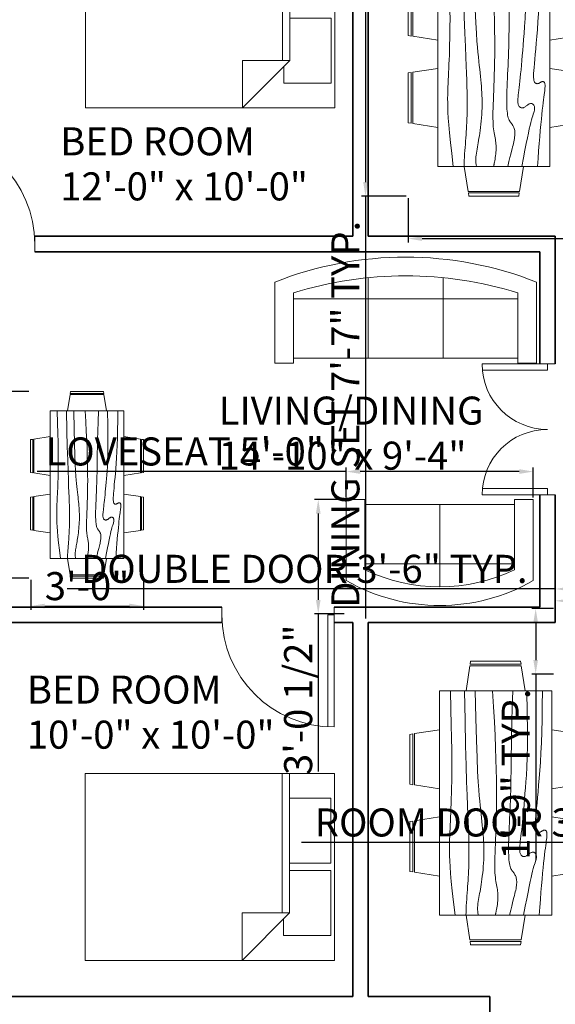
# Model space of a CAD drawing. Units: inches. Extents: x 3087 to 8148, y 1377 to 3709.
# Tile 3 of 6: x 3271 to 3443, y 1561 to 1877. Entities that reach past the tile are written whole.
import ezdxf

# ---------------------------------------------------------------- set-up
doc = ezdxf.new("R2010")
doc.units = ezdxf.units.IN
for name, color, linetype, lineweight, true_color in [('A-ANNO-DIMS', 244, 'Continuous', 18, 0x991b1e), ('A-AREA-IDEN', 244, 'Continuous', 18, 0x991b1e), ('A-DOOR', 146, 'Continuous', 18, 0x105689), ('A-WALL', 241, 'Continuous', 35, 0xf7abae)]:
    doc.layers.add(name, color=color, linetype=linetype, lineweight=lineweight, true_color=true_color)
doc.layers.add('A-FURN', color=8, linetype='Continuous', lineweight=18)
doc.styles.get("Standard").update_dxf_attribs({"font": 'arial.ttf'})
doc.dimstyles.new('ISO-25', dxfattribs={"dimtxt": 9, "dimasz": 4.5, "dimexe": 1.25, "dimexo": 0.625, "dimtad": 1, "dimdec": 0, "dimlunit": 3, "dimtxsty": 'Standard', "dimcen": 2.5, "dimadec": 0, "dimazin": 0, "dimtfac": 1, "dimtdec": 0, "dimtmove": 0, "dimatfit": 3, "dimfxl": 1, "dimarcsym": 0})

# ---------------------------------------------------------------- blocks, each defined once
blk = doc.blocks.new('Bed - Queen')
for p, q in [((0, -80.00003), (0, 0)), ((0, 0), (59.99999, 0)), ((59.99999, 0), (59.99999, -80.00003)), ((7.99999, -1.2), (28.79998, -1.2)), ((7.99999, -14.4), (7.99999, -1.2)), ((28.79998, -1.2), (28.79998, -14.4)), ((31.19999, -1.2), (51.99999, -1.2)), ((31.19999, -14.4), (31.19999, -1.2)), ((51.99999, -1.2), (51.99999, -16.4)), ((0, -14.4), (44.8, -14.4)), ((59.99999, -29.6), (44.8, -14.4)), ((44.8, -14.4), (44.8, -29.6)), ((44.8, -16.8), (0, -16.8)), ((51.99999, -16.4), (46.79936, -16.4)), ((44.8, -29.6), (59.99999, -29.6)), ((59.99999, -80.00003), (0, -80.00003))]:
    blk.add_line(p, q)
blk = doc.blocks.new('Dining Set - 36 x 72 in.')
for p, q in [((-22.2343, 26.00059), (-23.4847, 17.99762)), ((-22.2304, 26), (-5.7608, 26)), ((-22, 27.5), (-22.1562, 26.50042)), ((-5.8416, 26.5), (-22.1534, 26.5)), ((-22, 27.5), (-6, 27.5)), ((-5.8437, 26.49966), (-6, 27.5)), ((-4.5152, 17.99762), (-5.7655, 25.99926)), ((5.7657, 26.00059), (4.5153, 17.99762)), ((5.7696, 26), (22.2392, 26)), ((6, 27.5), (5.8438, 26.50042)), ((22.1584, 26.5), (5.8466, 26.5)), ((6, 27.5), (22, 27.5)), ((22.1563, 26.49966), (22, 27.5)), ((23.4848, 17.99762), (22.2345, 25.99926)), ((36, 18), (-36, 18)), ((-36, 18), (-36, -18)), ((36, -18), (36, 18)), ((-44.0006, 8.23428), (-35.9976, 9.48474)), ((44.0006, 8.23428), (35.9976, 9.48474)), ((-45.5, 8), (-44.5004, 8.15617)), ((-45.5, 8), (-45.5, -8)), ((-44.5, -8.15843), (-44.5, 8.15338)), ((-44, 8.23041), (-44, -8.23915)), ((44, 8.23041), (44, -8.23915)), ((44.5, -8.15843), (44.5, 8.15338)), ((45.5, 8), (44.5005, 8.15617)), ((45.5, 8), (45.5, -8)), ((-44.4997, -8.15631), (-45.5, -8)), ((-35.9976, -9.48476), (-43.9993, -8.2345)), ((35.9976, -9.48476), (43.9993, -8.2345)), ((44.4997, -8.15631), (45.5, -8)), ((-36, -18), (36, -18)), ((-22.2343, -26.0006), (-23.4847, -17.99762)), ((-4.5152, -17.99762), (-5.7655, -25.99928)), ((5.7657, -26.0006), (4.5153, -17.99762)), ((23.4848, -17.99762), (22.2345, -25.99928)), ((-22.2304, -26), (-5.7608, -26)), ((-22, -27.5), (-22.1562, -26.50044)), ((-5.8416, -26.5), (-22.1534, -26.5)), ((-22, -27.5), (-6, -27.5)), ((-5.8437, -26.49967), (-6, -27.5)), ((5.7696, -26), (22.2392, -26)), ((6, -27.5), (5.8438, -26.50044)), ((22.1584, -26.5), (5.8466, -26.5)), ((6, -27.5), (22, -27.5)), ((22.1563, -26.49967), (22, -27.5))]:
    blk.add_line(p, q)
for points in [[(-36, 15), (-31.1772, 14.97754), (-26.8079, 14.91406), (-22.8538, 14.81543), (-19.276, 14.6875), (-16.0362, 14.53613), (-13.0957, 14.36718), (-10.4159, 14.18652), (-7.9583, 14), (-5.6904, 13.81315), (-3.6035, 13.63021), (-1.6954, 13.45508), (0.0365, 13.29166), (1.5945, 13.14388), (2.9811, 13.01562), (4.1988, 12.9108), (5.25, 12.83333), (6.1393, 12.78613), (6.8802, 12.76823), (7.4883, 12.77767), (7.9792, 12.8125), (8.3685, 12.87077), (8.6719, 12.95052), (8.9049, 13.0498), (9.0833, 13.16666), (9.2205, 13.29899), (9.3216, 13.44401), (9.3895, 13.59879), (9.4271, 13.76041), (9.4373, 13.92594), (9.4232, 14.09245), (9.3875, 14.257), (9.3333, 14.41666), (9.2638, 14.56917), (9.1836, 14.71484), (9.0975, 14.85465), (9.0104, 14.98958), (8.9272, 15.1206), (8.8529, 15.2487), (8.7922, 15.37483), (8.75, 15.5), (8.7305, 15.62467), (8.7344, 15.74739), (8.7617, 15.86621), (8.8125, 15.97916), (8.8867, 16.08431), (8.9844, 16.17968), (9.1055, 16.26334), (9.25, 16.33333), (9.4189, 16.38802), (9.6172, 16.42708), (9.8506, 16.45052), (10.125, 16.45833), (10.4463, 16.45052), (10.8203, 16.42708), (11.2529, 16.38802), (11.75, 16.33333), (12.3184, 16.26318), (12.9694, 16.17838), (13.7151, 16.07991), (14.5677, 15.96875), (15.5395, 15.84586), (16.6426, 15.71224), (17.8893, 15.56884), (19.2917, 15.41666), (20.859, 15.25667), (22.5879, 15.08984), (24.4721, 14.91715), (26.5052, 14.73958), (28.6809, 14.5581), (30.9929, 14.3737), (33.4347, 14.18733), (36, 14)], [(-36, 10), (-28.9766, 10.14274), (-23.1725, 10.20442), (-18.4241, 10.19775), (-14.5677, 10.13541), (-11.4399, 10.03011), (-8.877, 9.89453), (-6.7154, 9.74137), (-4.7917, 9.58333), (-2.9698, 9.43082), (-1.2246, 9.28515), (0.4415, 9.14534), (2.026, 9.01041), (3.5266, 8.87939), (4.9408, 8.7513), (6.266, 8.62516), (7.5, 8.5), (8.6411, 8.37549), (9.6914, 8.2539), (10.6538, 8.13818), (11.5312, 8.03125), (12.3267, 7.93603), (13.043, 7.85547), (13.6831, 7.79248), (14.25, 7.75), (14.7471, 7.7303), (15.1797, 7.73307), (15.5537, 7.75732), (15.875, 7.80208), (16.1494, 7.86637), (16.3828, 7.94922), (16.5811, 8.04964), (16.75, 8.16666), (16.8944, 8.29915), (17.0143, 8.44531), (17.1089, 8.60319), (17.1771, 8.77083), (17.218, 8.94629), (17.2305, 9.1276), (17.2137, 9.31282), (17.1667, 9.5), (17.0895, 9.6875), (16.987, 9.875), (16.8649, 10.0625), (16.7292, 10.25), (16.5856, 10.4375), (16.4401, 10.625), (16.2985, 10.8125), (16.1667, 11), (16.05, 11.18733), (15.9518, 11.3737), (15.8752, 11.5581), (15.8229, 11.73958), (15.798, 11.91715), (15.8034, 12.08984), (15.842, 12.25667), (15.9167, 12.41666), (16.0295, 12.56836), (16.1784, 12.70833), (16.3605, 12.83268), (16.5729, 12.9375), (16.8127, 13.01888), (17.0768, 13.07291), (17.3625, 13.0957), (17.6667, 13.08333), (17.9894, 13.03312), (18.3418, 12.94726), (18.7382, 12.82918), (19.1927, 12.68229), (19.7195, 12.51001), (20.3327, 12.31575), (21.0465, 12.10294), (21.875, 11.875), (22.8357, 11.63354), (23.959, 11.37304), (25.2786, 11.08618), (26.8282, 10.76562), (28.6414, 10.40405), (30.752, 9.99414), (33.1936, 9.52856), (36, 9)], [(-36, 5.5), (-30.7157, 5.3348), (-26.069, 5.20963), (-21.9946, 5.11767), (-18.4271, 5.05208), (-15.3009, 5.00602), (-12.5508, 4.97265), (-10.1112, 4.94515), (-7.9167, 4.91666), (-5.909, 4.88167), (-4.0586, 4.83984), (-2.3429, 4.79215), (-0.7396, 4.73958), (0.7739, 4.6831), (2.22, 4.6237), (3.6213, 4.56233), (5, 4.5), (6.373, 4.43782), (7.7344, 4.3776), (9.0723, 4.32129), (10.375, 4.27083), (11.6309, 4.22819), (12.8281, 4.19531), (13.9551, 4.17415), (15, 4.16666), (15.954, 4.17448), (16.819, 4.19791), (17.6001, 4.23698), (18.3021, 4.29166), (18.9299, 4.36198), (19.4883, 4.44791), (19.9823, 4.54948), (20.4167, 4.66666), (20.7969, 4.79899), (21.1302, 4.94401), (21.4245, 5.09879), (21.6875, 5.26041), (21.9271, 5.42594), (22.1511, 5.59245), (22.3672, 5.757), (22.5834, 5.91666), (22.8065, 6.06868), (23.0404, 6.21093), (23.2879, 6.34147), (23.5521, 6.45833), (23.8358, 6.55957), (24.142, 6.64323), (24.4735, 6.70735), (24.8334, 6.75), (25.2235, 6.76969), (25.642, 6.76692), (26.0858, 6.74267), (26.5521, 6.69791), (27.0379, 6.63362), (27.5404, 6.55078), (28.0565, 6.45036), (28.5834, 6.33333), (29.1242, 6.19987), (29.7071, 6.04687), (30.3661, 5.87044), (31.1354, 5.66666), (32.0493, 5.43164), (33.142, 5.16146), (34.4475, 4.85221), (36, 4.5)], [(-36, -1), (-30.7915, -0.6591), (-26.0195, -0.38216), (-21.6519, -0.16284), (-17.6563, 0.00521), (-14.0005, 0.12833), (-10.6523, 0.21289), (-7.5796, 0.26522), (-4.75, 0.29166), (-2.134, 0.29793), (0.2878, 0.28711), (2.5317, 0.26163), (4.6146, 0.22396), (6.5529, 0.17651), (8.3633, 0.12174), (10.0623, 0.06209), (11.6667, 0), (13.1899, -0.06201), (14.6341, -0.1211), (15.9982, -0.17432), (17.2813, -0.21875), (18.4823, -0.25147), (19.6003, -0.26953), (20.6343, -0.27002), (21.5834, -0.25), (22.4481, -0.20768), (23.2357, -0.14584), (23.9549, -0.06836), (24.6146, 0.02083), (25.2235, 0.11784), (25.7904, 0.21875), (26.3241, 0.31966), (26.8334, 0.41666), (27.3265, 0.50618), (27.8099, 0.58593), (28.2894, 0.65397), (28.7709, 0.70833), (29.2601, 0.74707), (29.763, 0.76823), (30.2855, 0.76985), (30.8334, 0.75), (31.4088, 0.70784), (31.9994, 0.64713), (32.589, 0.57275), (33.1615, 0.48958), (33.7008, 0.4025), (34.1908, 0.3164), (34.6153, 0.23616), (34.9584, 0.16666), (35.2099, 0.11165), (35.3848, 0.07031), (35.504, 0.04069), (35.5886, 0.02083), (35.6594, 0.00879), (35.7377, 0.0026), (35.8442, 0.00032), (36, 0)], [(-36, -6.5), (-27.1843, -6.31267), (-20.084, -6.1263), (-14.469, -5.9419), (-10.1094, -5.76042), (-6.7752, -5.58285), (-4.2363, -5.41016), (-2.2629, -5.24333), (-0.625, -5.08334), (0.8708, -4.93099), (2.2715, -4.78646), (3.5872, -4.64974), (4.8281, -4.52084), (6.0046, -4.39974), (7.127, -4.28646), (8.2053, -4.18099), (9.25, -4.08334), (10.2705, -3.99382), (11.2734, -3.91407), (12.2647, -3.84603), (13.25, -3.79167), (14.2354, -3.75293), (15.2266, -3.73177), (16.2295, -3.73015), (17.25, -3.75), (18.2912, -3.79248), (19.3451, -3.85547), (20.4009, -3.93604), (21.4479, -4.03125), (22.4754, -4.13819), (23.4727, -4.25391), (24.4289, -4.37549), (25.3334, -4.5), (26.1785, -4.62492), (26.9694, -4.74935), (27.7145, -4.87281), (28.4219, -4.99479), (29.1, -5.11483), (29.7572, -5.23242), (30.4016, -5.34709), (31.0417, -5.45834), (31.6837, -5.56437), (32.3262, -5.65821), (32.9658, -5.73153), (33.599, -5.77604), (34.2224, -5.78345), (34.8327, -5.74545), (35.4264, -5.65373), (36, -5.5)], [(-36, -10), (-26.4022, -9.81299), (-18.4675, -9.62891), (-11.9839, -9.45069), (-6.7396, -9.28125), (-2.5226, -9.12354), (0.8789, -8.98047), (3.6769, -8.85498), (6.0833, -8.75), (8.2767, -8.66765), (10.3021, -8.60677), (12.1712, -8.56543), (13.8958, -8.54167), (15.4876, -8.53353), (16.9583, -8.53907), (18.3197, -8.55632), (19.5834, -8.58334), (20.7616, -8.61841), (21.8685, -8.66081), (22.9188, -8.71004), (23.9271, -8.76563), (24.9081, -8.82707), (25.8763, -8.89388), (26.8465, -8.96558), (27.8334, -9.04167), (28.8474, -9.12118), (29.8828, -9.20117), (30.93, -9.27824), (31.9792, -9.34896), (33.0205, -9.40991), (34.0443, -9.45768), (35.0407, -9.48885), (36, -9.5)], [(-36, -14.5), (-30.0881, -14.33513), (-25.0332, -14.21224), (-20.7312, -14.12647), (-17.0781, -14.07292), (-13.97, -14.04671), (-11.3027, -14.04297), (-8.9724, -14.05681), (-6.875, -14.08334), (-4.9224, -14.11833), (-3.0905, -14.16016), (-1.3709, -14.20785), (0.2448, -14.26042), (1.7647, -14.3169), (3.1973, -14.3763), (4.5507, -14.43767), (5.8333, -14.5), (7.0554, -14.5621), (8.235, -14.62175), (9.3922, -14.67652), (10.5469, -14.72396), (11.7192, -14.76164), (12.929, -14.78711), (14.1965, -14.79794), (15.5417, -14.79167), (16.9933, -14.76424), (18.6152, -14.70508), (20.4804, -14.60197), (22.6615, -14.44271), (25.2312, -14.21509), (28.2624, -13.9069), (31.8277, -13.50594), (36, -13)]]:
    blk.add_lwpolyline(points)
blk = doc.blocks.new('Sofa - Roundback 7 ft.')
for p, q in [((-12.00002, -32.4421), (-12.00003, -6.5971)), ((11.99997, -32.4421), (11.99998, -6.5971)), ((-36.000027, -34), (-36.000027, -11.4696)), ((35.99998, -34), (35.99998, -11.4696)), ((-35.999844, -13.3819), (35.9998, -13.3819)), ((-36.000027, -32.4421), (35.99998, -32.4421))]:
    blk.add_line(p, q)
for points in [[(-36.000027, -34), (-42.000027, -34), (-42.000027, -8)], [(41.99998, -8), (41.99998, -34), (35.99998, -34)]]:
    blk.add_lwpolyline(points)
for centre, radius, start, end in [((0, -114.25), 114.25, 68.43141, 111.5686), ((-0.00001, -127.1968), 121.1968, 72.72033, 107.2797)]:
    blk.add_arc(centre, radius, start, end)
blk = doc.blocks.new('Sofa - Roundback Loveseat 5 ft.')
for p, q in [((0, -32.44198), (0, -5.99998)), ((-24, -33.99998), (-24, -11.46958)), ((24.00004, -33.99998), (24.00004, -11.46958)), ((-23.9998, -13.38178), (23.99986, -13.38178)), ((-24, -32.44198), (24.00004, -32.44198))]:
    blk.add_line(p, q)
for points in [[(-24, -33.99998), (-30, -33.99998), (-30, -7.99998)], [(30.00004, -7.99998), (30.00004, -33.99998), (24.00004, -33.99998)]]:
    blk.add_lwpolyline(points)
for centre, radius, start, end in [((0, -60.24998), 60.24998, 60.13715, 119.8628), ((0, -61.38438), 55.38444, 64.32083, 115.6792)]:
    blk.add_arc(centre, radius, start, end)
blk = doc.blocks.new('*D19')
at = {"layer": 'A-ANNO-DIMS', "color": 0, "lineweight": -2, "transparency": 16777216}
for p, q in [((3442.82, 1703.84), (3442.82, 1689.71)), ((3630.82, 1703.84), (3630.82, 1689.71)), ((3447.32, 1690.96), (3626.32, 1690.96))]:
    blk.add_line(p, q, dxfattribs=at)
at = {"layer": 'A-ANNO-DIMS', "color": 0, "transparency": 16777216}
for points in [[(3447.32, 1691.71), (3447.32, 1690.21), (3442.82, 1690.96)], [(3626.32, 1691.71), (3626.32, 1690.21), (3630.82, 1690.96)]]:
    blk.add_solid(points, dxfattribs=at)
at = {"layer": 'Defpoints', "color": 0, "transparency": 16777216}
for p in [(3442.82, 1704.46), (3630.82, 1704.46), (3630.82, 1690.96)]:
    blk.add_point(p, dxfattribs=at)
at = {"layer": 'A-ANNO-DIMS', "color": 0, "transparency": 16777216, "insert": (3536.82, 1696.18), "char_height": 9, "attachment_point": 5}
blk.add_mtext('15\'-8"', dxfattribs=at)
blk = doc.blocks.new('DOOR-SINGLE-36IN')
for p, q in [((0, 2), (36, 2)), ((36, 0), (36, 2)), ((0, 0), (36, 0))]:
    blk.add_line(p, q)
blk.add_arc((36, 0), 36, 90, 180)
blk = doc.blocks.new('DOOR-DOUBLE-42IN')
for p, q in [((0, 21), (0, 0)), ((2, 21), (2, 0)), ((40, 21), (40, 0)), ((42, 21), (42, 0)), ((0, 0), (2, 0)), ((42, 0), (40, 0))]:
    blk.add_line(p, q)
for centre, start, end in [((0, 0), 0, 90), ((42, 0), 90, 180)]:
    blk.add_arc(centre, 21, start, end)
blk = doc.blocks.new('*D29')
at = {"layer": 'A-ANNO-DIMS', "color": 0, "lineweight": -2, "transparency": 16777216}
for p, q in [((3505.32, 1613.36), (3361.36, 1613.36)), ((3505.32, 1608.59), (3505.32, 1614.61)), ((3536.82, 1613.36), (3509.82, 1613.36)), ((3541.32, 1608.59), (3541.32, 1614.61))]:
    blk.add_line(p, q, dxfattribs=at)
at = {"layer": 'A-ANNO-DIMS', "color": 0, "transparency": 16777216}
for points in [[(3509.82, 1614.11), (3509.82, 1612.61), (3505.32, 1613.36)], [(3536.82, 1614.11), (3536.82, 1612.61), (3541.32, 1613.36)]]:
    blk.add_solid(points, dxfattribs=at)
at = {"layer": 'Defpoints', "color": 0, "transparency": 16777216}
for p in [(3505.32, 1613.36), (3505.32, 1607.96), (3541.32, 1607.96)]:
    blk.add_point(p, dxfattribs=at)
at = {"layer": 'A-ANNO-DIMS', "color": 0, "transparency": 16777216, "insert": (3431.09, 1618.65), "char_height": 9, "attachment_point": 5}
blk.add_mtext('ROOM DOOR 3\'-0" TYP.', dxfattribs=at)
blk = doc.blocks.new('*D41')
at = {"layer": 'A-ANNO-DIMS', "color": 0, "lineweight": -2, "transparency": 16777216}
for p, q in [((3394.96, 1911.86), (3380.68, 1911.86)), ((3381.93, 1907.36), (3381.93, 1825.36)), ((3394.96, 1820.86), (3380.68, 1820.86)), ((3381.93, 1820.86), (3381.93, 1685.25))]:
    blk.add_line(p, q, dxfattribs=at)
at = {"layer": 'A-ANNO-DIMS', "color": 0, "transparency": 16777216}
for points in [[(3381.18, 1907.36), (3382.68, 1907.36), (3381.93, 1911.86)], [(3381.18, 1825.36), (3382.68, 1825.36), (3381.93, 1820.86)]]:
    blk.add_solid(points, dxfattribs=at)
at = {"layer": 'Defpoints', "color": 0, "transparency": 16777216}
for p in [(3395.58, 1911.86), (3381.93, 1820.86), (3395.58, 1820.86)]:
    blk.add_point(p, dxfattribs=at)
at = {"layer": 'A-ANNO-DIMS', "color": 0, "transparency": 16777216, "insert": (3376.65, 1750.81), "char_height": 9, "attachment_point": 5, "rotation": 90}
blk.add_mtext('DINING SET 7\'-7" TYP.', dxfattribs=at)
blk = doc.blocks.new('*D42')
at = {"layer": 'A-ANNO-DIMS', "color": 0, "lineweight": -2, "transparency": 16777216}
for p, q in [((3395.58, 1820.23), (3395.58, 1805.96)), ((3450.58, 1820.23), (3450.58, 1805.96)), ((3400.08, 1807.21), (3446.08, 1807.21)), ((3450.58, 1807.21), (3511.55, 1807.21))]:
    blk.add_line(p, q, dxfattribs=at)
at = {"layer": 'A-ANNO-DIMS', "color": 0, "transparency": 16777216}
for points in [[(3400.08, 1807.96), (3400.08, 1806.46), (3395.58, 1807.21)], [(3446.08, 1807.96), (3446.08, 1806.46), (3450.58, 1807.21)]]:
    blk.add_solid(points, dxfattribs=at)
at = {"layer": 'Defpoints', "color": 0, "transparency": 16777216}
for p in [(3395.58, 1820.86), (3450.58, 1820.86), (3450.58, 1807.21)]:
    blk.add_point(p, dxfattribs=at)
at = {"layer": 'A-ANNO-DIMS', "color": 0, "transparency": 16777216, "insert": (3483.32, 1812.34), "char_height": 9, "attachment_point": 5}
blk.add_mtext('4\'-7" TYP.', dxfattribs=at)
blk = doc.blocks.new('*D43')
at = {"layer": 'A-ANNO-DIMS', "color": 0, "lineweight": -2, "transparency": 16777216}
for p, q in [((3273.87, 1758.14), (3264.27, 1758.14)), ((3265.52, 1753.64), (3265.52, 1702.76)), ((3273.87, 1698.26), (3264.27, 1698.26)), ((3265.52, 1698.26), (3265.52, 1593.59))]:
    blk.add_line(p, q, dxfattribs=at)
at = {"layer": 'A-ANNO-DIMS', "color": 0, "transparency": 16777216}
for points in [[(3264.77, 1753.64), (3266.27, 1753.64), (3265.52, 1758.14)], [(3264.77, 1702.76), (3266.27, 1702.76), (3265.52, 1698.26)]]:
    blk.add_solid(points, dxfattribs=at)
at = {"layer": 'Defpoints', "color": 0, "transparency": 16777216}
for p in [(3274.5, 1758.14), (3265.52, 1698.26), (3274.5, 1698.26)]:
    blk.add_point(p, dxfattribs=at)
at = {"layer": 'A-ANNO-DIMS', "color": 0, "transparency": 16777216, "insert": (3260.24, 1643.68), "char_height": 9, "attachment_point": 5, "rotation": 90}
blk.add_mtext('DINING SET 5\'-0"', dxfattribs=at)
blk = doc.blocks.new('*D44')
at = {"layer": 'A-ANNO-DIMS', "color": 0, "lineweight": -2, "transparency": 16777216}
for p, q in [((3274.5, 1697.64), (3274.5, 1688.03)), ((3310.69, 1697.64), (3310.69, 1688.03)), ((3279, 1689.28), (3306.19, 1689.28))]:
    blk.add_line(p, q, dxfattribs=at)
at = {"layer": 'A-ANNO-DIMS', "color": 0, "transparency": 16777216}
for points in [[(3279, 1690.03), (3279, 1688.53), (3274.5, 1689.28)], [(3306.19, 1690.03), (3306.19, 1688.53), (3310.69, 1689.28)]]:
    blk.add_solid(points, dxfattribs=at)
at = {"layer": 'Defpoints', "color": 0, "transparency": 16777216}
for p in [(3274.5, 1698.26), (3310.69, 1698.26), (3310.69, 1689.28)]:
    blk.add_point(p, dxfattribs=at)
at = {"layer": 'A-ANNO-DIMS', "color": 0, "transparency": 16777216, "insert": (3292.59, 1694.5), "char_height": 9, "attachment_point": 5}
blk.add_mtext('3\'-0"', dxfattribs=at)
blk = doc.blocks.new('*D49')
at = {"layer": 'A-ANNO-DIMS', "color": 0, "lineweight": -2, "transparency": 16777216}
for p, q in [((3442.82, 1694.76), (3286.25, 1694.76)), ((3442.82, 1689.09), (3442.82, 1696.01)), ((3480.32, 1694.76), (3447.32, 1694.76)), ((3484.82, 1689.09), (3484.82, 1696.01))]:
    blk.add_line(p, q, dxfattribs=at)
at = {"layer": 'A-ANNO-DIMS', "color": 0, "transparency": 16777216}
for points in [[(3447.32, 1695.51), (3447.32, 1694.01), (3442.82, 1694.76)], [(3480.32, 1695.51), (3480.32, 1694.01), (3484.82, 1694.76)]]:
    blk.add_solid(points, dxfattribs=at)
at = {"layer": 'Defpoints', "color": 0, "transparency": 16777216}
for p in [(3442.82, 1694.76), (3442.82, 1688.46), (3484.82, 1688.46)]:
    blk.add_point(p, dxfattribs=at)
at = {"layer": 'A-ANNO-DIMS', "color": 0, "transparency": 16777216, "insert": (3362.28, 1700.05), "char_height": 9, "attachment_point": 5}
blk.add_mtext('DOUBLE DOOR 3\'-6" TYP.', dxfattribs=at)
blk = doc.blocks.new('*D50')
at = {"layer": 'A-ANNO-DIMS', "color": 0, "lineweight": -2, "transparency": 16777216}
for p, q in [((3442.19, 1688.46), (3435.27, 1688.46)), ((3436.52, 1683.96), (3436.52, 1671.96)), ((3442.19, 1667.46), (3435.27, 1667.46)), ((3436.52, 1667.46), (3436.52, 1607.7))]:
    blk.add_line(p, q, dxfattribs=at)
at = {"layer": 'A-ANNO-DIMS', "color": 0, "transparency": 16777216}
for points in [[(3435.77, 1683.96), (3437.27, 1683.96), (3436.52, 1688.46)], [(3435.77, 1671.96), (3437.27, 1671.96), (3436.52, 1667.46)]]:
    blk.add_solid(points, dxfattribs=at)
at = {"layer": 'Defpoints', "color": 0, "transparency": 16777216}
for p in [(3442.82, 1688.46), (3436.52, 1667.46), (3442.82, 1667.46)]:
    blk.add_point(p, dxfattribs=at)
at = {"layer": 'A-ANNO-DIMS', "color": 0, "transparency": 16777216, "insert": (3431.3, 1635.33), "char_height": 9, "attachment_point": 5, "rotation": 90}
blk.add_mtext('1\'-9" TYP.', dxfattribs=at)
blk = doc.blocks.new('*D53')
at = {"layer": 'A-ANNO-DIMS', "color": 0, "lineweight": -2, "transparency": 16777216}
for p, q in [((3375.76, 1732.44), (3276.61, 1732.44)), ((3375.76, 1724.07), (3375.76, 1733.69)), ((3431.26, 1732.44), (3380.26, 1732.44)), ((3435.76, 1724.07), (3435.76, 1733.69))]:
    blk.add_line(p, q, dxfattribs=at)
at = {"layer": 'A-ANNO-DIMS', "color": 0, "transparency": 16777216}
for points in [[(3380.26, 1733.19), (3380.26, 1731.69), (3375.76, 1732.44)], [(3431.26, 1733.19), (3431.26, 1731.69), (3435.76, 1732.44)]]:
    blk.add_solid(points, dxfattribs=at)
at = {"layer": 'Defpoints', "color": 0, "transparency": 16777216}
for p in [(3375.76, 1732.44), (3375.76, 1723.44), (3435.76, 1723.44)]:
    blk.add_point(p, dxfattribs=at)
at = {"layer": 'A-ANNO-DIMS', "color": 0, "transparency": 16777216, "insert": (3323.93, 1737.72), "char_height": 9, "attachment_point": 5}
blk.add_mtext('LOVESEAT 5\'-0"', dxfattribs=at)
blk = doc.blocks.new('*D54')
at = {"layer": 'A-ANNO-DIMS', "color": 0, "lineweight": -2, "transparency": 16777216}
for p, q in [((3375.13, 1723.44), (3365.51, 1723.44)), ((3366.76, 1718.94), (3366.76, 1691.27)), ((3375.13, 1686.77), (3365.51, 1686.77)), ((3366.76, 1686.77), (3366.76, 1636.13))]:
    blk.add_line(p, q, dxfattribs=at)
at = {"layer": 'A-ANNO-DIMS', "color": 0, "transparency": 16777216}
for points in [[(3366.01, 1718.94), (3367.51, 1718.94), (3366.76, 1723.44)], [(3366.01, 1691.27), (3367.51, 1691.27), (3366.76, 1686.77)]]:
    blk.add_solid(points, dxfattribs=at)
at = {"layer": 'Defpoints', "color": 0, "transparency": 16777216}
for p in [(3375.76, 1723.44), (3366.76, 1686.77), (3375.76, 1686.77)]:
    blk.add_point(p, dxfattribs=at)
at = {"layer": 'A-ANNO-DIMS', "color": 0, "transparency": 16777216, "insert": (3361.48, 1659.2), "char_height": 9, "attachment_point": 5, "rotation": 90}
blk.add_mtext('3\'-0 1/2"', dxfattribs=at)

msp = doc.modelspace()

# ---------------------------------------------------------------- linework, layer by layer
at = {"layer": 'A-DOOR'}
for p, q in [((3275.82, 1802.96), (3275.82, 1807.96)), ((3442.82, 1766.96), (3437.82, 1766.96)), ((3442.82, 1724.96), (3437.82, 1724.96)), ((3335.82, 1683.96), (3335.82, 1688.96)), ((3371.82, 1683.96), (3371.82, 1688.96))]:
    msp.add_line(p, q, dxfattribs=at)
at = {"layer": 'A-WALL'}
for p, q in [((3377.82, 1807.96), (3377.82, 1927.96)), ((3382.82, 1807.96), (3382.82, 1927.96)), ((3275.82, 1807.96), (3377.82, 1807.96)), ((3382.82, 1807.96), (3442.82, 1807.96)), ((3442.82, 1766.96), (3442.82, 1807.96)), ((3275.82, 1802.96), (3437.82, 1802.96)), ((3437.82, 1766.96), (3437.82, 1802.96)), ((3437.82, 1688.96), (3437.82, 1724.96)), ((3442.82, 1683.96), (3442.82, 1724.96)), ((3257.82, 1688.96), (3335.82, 1688.96)), ((3371.82, 1688.96), (3437.82, 1688.96)), ((3257.82, 1683.96), (3335.82, 1683.96)), ((3371.82, 1683.96), (3377.82, 1683.96)), ((3377.82, 1563.96), (3377.82, 1683.96)), ((3382.82, 1563.96), (3382.82, 1683.96)), ((3382.82, 1683.96), (3442.82, 1683.96)), ((3257.82, 1563.96), (3377.82, 1563.96)), ((3382.82, 1563.96), (3421.82, 1563.96)), ((3421.82, 1558.96), (3421.82, 1563.96))]:
    msp.add_line(p, q, dxfattribs=at)

# ---------------------------------------------------------------- block references
at = {"layer": 'A-DOOR'}
for name, p, rotation in [('DOOR-SINGLE-36IN', (3239.82, 1841.46), 270.0000000000006), ('DOOR-DOUBLE-42IN', (3440.32, 1724.96), 90.000000000002), ('DOOR-SINGLE-36IN', (3371.82, 1650.46), 89.9999999999992)]:
    msp.add_blockref(name, p, dxfattribs=dict(at, rotation=rotation))
at = {"layer": 'A-FURN'}
for name, p, rotation in [('Dining Set - 36 x 72 in.', (3423.08, 1866.36), 269.9999999999999), ('Bed - Queen', (3372.09, 1909.14), 270), ('Sofa - Roundback Loveseat 5 ft.', (3405.76, 1689.44), 180), ('Dining Set - 36 x 72 in.', (3423.66, 1626.1), 269.9999999999999), ('Bed - Queen', (3371.97, 1635.57), 270)]:
    msp.add_blockref(name, p, dxfattribs=dict(at, rotation=rotation))
msp.add_blockref('Sofa - Roundback 7 ft.', (3394.81, 1801.26), dxfattribs=at)
at = {"layer": 'A-FURN', "xscale": 0.6580386597318908, "yscale": 0.6580386597318908, "zscale": 0.6580386597318908, "rotation": 269.9999999999999}
msp.add_blockref('Dining Set - 36 x 72 in.', (3292.59, 1728.2), dxfattribs=at)

# ---------------------------------------------------------------- texts
at = {"layer": 'A-AREA-IDEN'}
for s, p in [('BED ROOM ', (3283.98, 1833.92)), ('12\'-0" x 10\'-0"', (3283.98, 1819.46)), ('LIVING/DINING', (3334.83, 1747.5)), ('14\'-10" x 9\'-4"', (3334.83, 1733.04)), ('BED ROOM ', (3273.27, 1657.96)), ('10\'-0" x 10\'-0"', (3273.27, 1643.5))]:
    msp.add_text(s, height=9, dxfattribs=at).set_placement(p)

# ---------------------------------------------------------------- dimensions: what is measured, and where the dimension line sits
at = {"layer": 'A-ANNO-DIMS'}
for base, p1, p2, angle, text, picture, middle in [((3381.93, 1820.86), (3395.58, 1911.86), (3395.58, 1820.86), 270, 'DINING SET <> TYP.', '*D41', (3376.65, 1750.81)), ((3265.52, 1698.26), (3274.5, 1758.14), (3274.5, 1698.26), 270, 'DINING SET <>', '*D43', (3260.24, 1643.68)), ((3375.76, 1732.44), (3435.76, 1723.44), (3375.76, 1723.44), 180, 'LOVESEAT <>', '*D53', (3323.93, 1737.72)), ((3442.82, 1694.76), (3484.82, 1688.46), (3442.82, 1688.46), 180, 'DOUBLE DOOR <> TYP.', '*D49', (3362.28, 1700.05)), ((3436.52, 1667.46), (3442.82, 1688.46), (3442.82, 1667.46), 270, '<> TYP.', '*D50', (3431.3, 1635.33)), ((3505.32, 1613.36), (3541.32, 1607.96), (3505.32, 1607.96), 180, 'ROOM DOOR <> TYP.', '*D29', (3431.09, 1618.65))]:
    dim = msp.add_linear_dim(base=base, p1=p1, p2=p2, angle=angle, text=text, dimstyle='ISO-25', override={"dimdec": 1, "dimlfac": 1, "dimrnd": 0, "dimzin": 1, "dimdsep": 46, "dimlunit": 4, "dimfrac": 2}, dxfattribs=at)
    dim.commit()
    dim.dimension.update_dxf_attribs({"geometry": picture, "text_midpoint": middle})
dim = msp.add_linear_dim(base=(3450.58, 1807.21), p1=(3395.58, 1820.86), p2=(3450.58, 1820.86), text='<> TYP.', dimstyle='ISO-25', override={"dimdec": 1, "dimlfac": 1, "dimrnd": 0, "dimzin": 1, "dimdsep": 46, "dimlunit": 4, "dimfrac": 2}, dxfattribs=at)
dim.commit()
dim.dimension.update_dxf_attribs({"geometry": '*D42', "text_midpoint": (3483.32, 1812.34)})
dim = msp.add_linear_dim(base=(3366.76, 1686.77), p1=(3375.76, 1723.44), p2=(3375.76, 1686.77), angle=270, dimstyle='ISO-25', override={"dimdec": 1, "dimlfac": 1, "dimrnd": 0, "dimzin": 1, "dimdsep": 46, "dimlunit": 4, "dimfrac": 2}, dxfattribs=at)
dim.commit()
dim.dimension.update_dxf_attribs({"geometry": '*D54', "text_midpoint": (3361.48, 1659.2)})
for base, p1, p2, override, picture, middle in [((3630.82, 1690.96), (3442.82, 1704.46), (3630.82, 1704.46), {"dimclrd": 0, "dimclre": 0, "dimclrt": 0}, '*D19', (3536.82, 1696.18)), ((3310.69, 1689.28), (3274.5, 1698.26), (3310.69, 1698.26), {"dimdec": 1, "dimlfac": 1, "dimrnd": 0, "dimzin": 1, "dimdsep": 46, "dimlunit": 4, "dimfrac": 2}, '*D44', (3292.59, 1694.5))]:
    dim = msp.add_linear_dim(base=base, p1=p1, p2=p2, dimstyle='ISO-25', override=override, dxfattribs=at)
    dim.commit()
    dim.dimension.update_dxf_attribs({"geometry": picture, "text_midpoint": middle})

doc.saveas('drawing.dxf')
